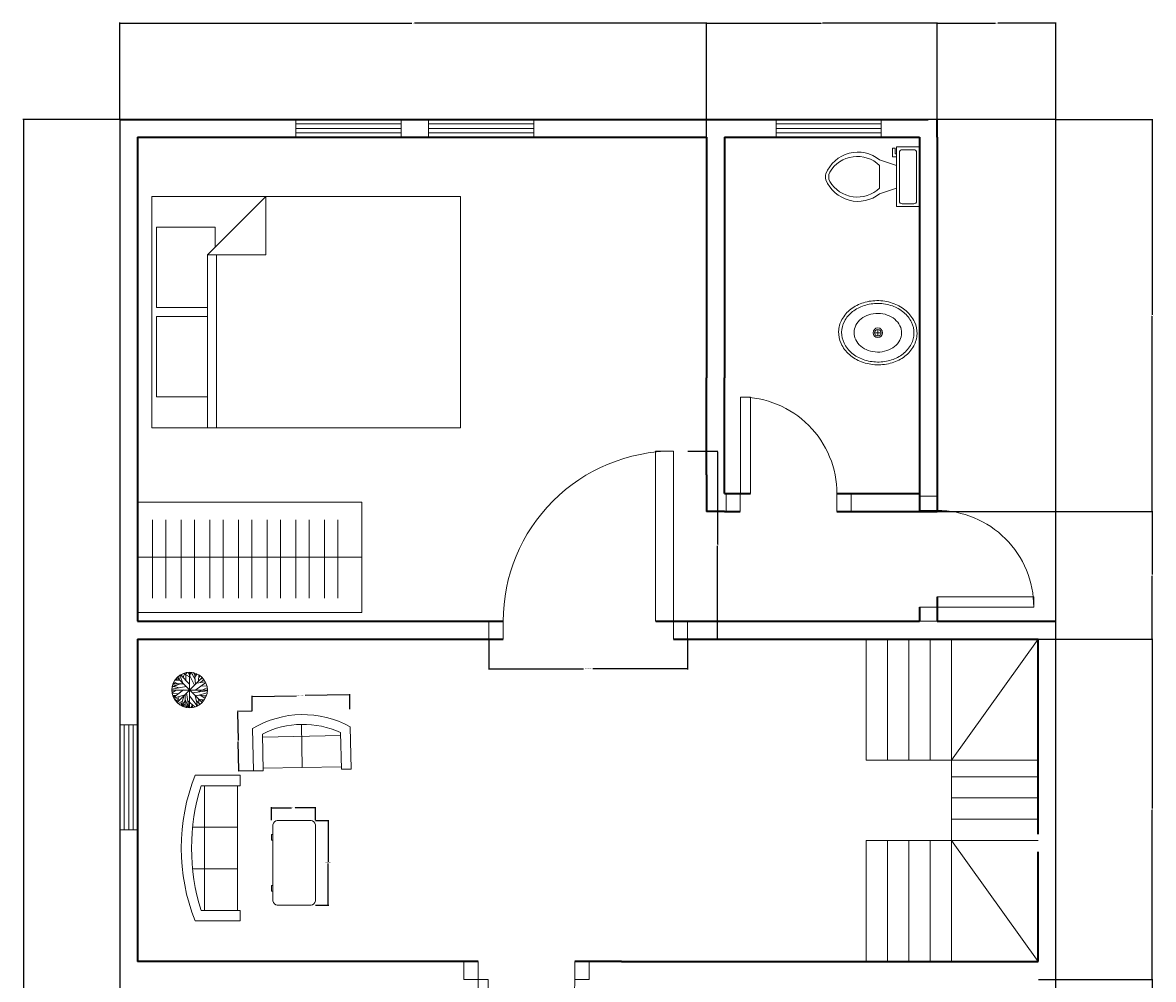
# Model space of a CAD drawing. Units: feet. Extents: x 2306 to 3052, y 829 to 1424.
# Tile 5 of 5: x 2733 to 3052, y 1154 to 1424. Entities that reach past the tile are written whole.
import ezdxf

# ---------------------------------------------------------------- set-up
doc = ezdxf.new("R2010")
doc.units = ezdxf.units.FT
for name, color, linetype, lineweight in [('A-ANNO-DIMS', 2, 'Continuous', 18), ('A-DOOR', 3, 'Continuous', 18), ('A-FLOR-FIXT', 9, 'Continuous', 18), ('A-FLOR-OTLN', 7, 'Continuous', 25), ('A-FLOR-STRS', 7, 'Continuous', 18), ('A-FURN', 8, 'Continuous', 13), ('A-GLAZ', 4, 'Continuous', 18), ('A-WALL', 7, 'Continuous', 35), ('L-PLNT', 94, 'Continuous', 13)]:
    doc.layers.add(name, color=color, linetype=linetype, lineweight=lineweight)
doc.styles.get("Standard").update_dxf_attribs({"font": 'arial.ttf'})
doc.dimstyles.get("Standard").update_dxf_attribs({"dimtxt": 0.18, "dimasz": 0.18, "dimexe": 0.18, "dimexo": 0.0625, "dimgap": 0.09, "dimtad": 0, "dimtih": 1, "dimtoh": 1, "dimdec": 4, "dimzin": 0, "dimdsep": 46, "dimlunit": 4, "dimtxsty": 'Standard', "dimcen": 0.09, "dimadec": 0, "dimazin": 0, "dimtfac": 1, "dimtdec": 4, "dimtofl": 0, "dimtmove": 0, "dimatfit": 3, "dimfxl": 1, "dimtolj": 1, "dimtzin": 0, "dimarcsym": 0})

# ---------------------------------------------------------------- blocks, each defined once
blk = doc.blocks.new('Window - Wood Frame 36 in. Wide plan')
for p, q in [((0, 6), (0, 0)), ((0, 4.5), (36, 4.5)), ((36, 6), (36, 0)), ((0, 3), (36, 3)), ((0, 1.5), (36, 1.5))]:
    blk.add_line(p, q)
blk = doc.blocks.new('Bed - Queen')
for p, q in [((0, -80.00003), (0, 0)), ((0, 0), (59.99999, 0)), ((59.99999, 0), (59.99999, -80.00003)), ((7.99999, -1.2), (28.79998, -1.2)), ((7.99999, -14.4), (7.99999, -1.2)), ((28.79998, -1.2), (28.79998, -14.4)), ((31.19999, -1.2), (51.99999, -1.2)), ((31.19999, -14.4), (31.19999, -1.2)), ((51.99999, -1.2), (51.99999, -16.4)), ((0, -14.4), (44.8, -14.4)), ((59.99999, -29.6), (44.8, -14.4)), ((44.8, -14.4), (44.8, -29.6)), ((44.8, -16.8), (0, -16.8)), ((51.99999, -16.4), (46.79936, -16.4)), ((44.8, -29.6), (59.99999, -29.6)), ((59.99999, -80.00003), (0, -80.00003))]:
    blk.add_line(p, q)
blk = doc.blocks.new('Toilet - top')
for p, q in [((9.5, -6), (9.5, -2)), ((-10, -8.5), (-8, -8.5)), ((-10, -9.5), (-10, -8.5)), ((-7, -9.5), (-10, -9.5)), ((-8, -8.5), (-8, -8)), ((-7, -8), (-7, -9.5)), ((-4, -8), (-6, -14)), ((4, -8), (6, -14)), ((4, -14), (-4, -14))]:
    blk.add_line(p, q)
blk.add_lwpolyline([(10.5, -8), (10.5, 0), (-10.5, 0), (-10.5, -8)], close=True)
for points in [[(-9.5, -2), (-9.5, -6)], [(8.5, -1), (-8.5, -1)], [(-8.5, -7), (8.5, -7)]]:
    blk.add_lwpolyline(points)
for centre, radius, start, end in [((-8.62, -1.88), 0.884, 81.8699, 188.1301), ((8.62, -1.88), 0.884, 351.8699, 98.1301), ((-8.62, -6.12), 0.884, 171.8699, 278.1301), ((8.62, -6.12), 0.884, 261.8699, 8.1301), ((3.52, -21.58), 12.17, 141.4691, 247.9714), ((4.2, -21.82), 11.33, 136.3677, 238.9468), ((-3.52, -21.58), 12.17, 292.0284, 38.5307), ((-4.2, -21.82), 11.33, 301.053, 43.6321), ((0, -27.88), 4, 245.7318, 294.2682), ((0, -29), 4, 254.8605, 285.1395)]:
    blk.add_arc(centre, radius, start, end)
blk = doc.blocks.new('Sink - Oval top')
for p, q in [((-1, 0), (1, 0)), ((0, 1), (0, -1))]:
    blk.add_line(p, q)
for points in [[(-12.23, 0.39, 0.117634), (-11.46, -3.36, 0.104469), (-8.88, -6.8, 0.090016), (-5.08, -9.07, 0.08192), (-0.32, -10.02, 0.08192), (4.49, -9.38, 0.090016), (8.42, -7.36, 0.104469), (11.22, -4.09, 0.117634), (12.23, -0.39, 0.117634), (11.46, 3.36, 0.104469), (8.88, 6.8, 0.090016), (5.08, 9.07, 0.08192), (0.32, 10.02, 0.08192), (-4.49, 9.38, 0.090016), (-8.42, 7.36, 0.104469), (-11.22, 4.09, 0.117634)], [(-11.29, 0.16, 0.118622), (-10.52, -3.25, 0.104678), (-8.07, -6.36, 0.089562), (-4.54, -8.37, 0.081185), (-0.13, -9.15, 0.081185), (4.3, -8.49, 0.089562), (7.89, -6.58, 0.104678), (10.42, -3.55, 0.118622), (11.29, -0.16, 0.118622), (10.52, 3.25, 0.104678), (8.07, 6.36, 0.089562), (4.54, 8.37, 0.081185), (0.13, 9.15, 0.081185), (-4.3, 8.49, 0.089562), (-7.89, 6.58, 0.104678), (-10.42, 3.55, 0.118622)], [(-7.42, 0.08, 0.118283), (-6.91, -2.17, 0.104607), (-5.29, -4.21, 0.089718), (-2.97, -5.53, 0.081436), (-0.07, -6.04, 0.081436), (2.84, -5.59, 0.089718), (5.2, -4.33, 0.104607), (6.86, -2.32, 0.118283), (7.42, -0.08, 0.118283), (6.91, 2.17, 0.104607), (5.29, 4.21, 0.089718), (2.97, 5.53, 0.081436), (0.07, 6.04, 0.081436), (-2.84, 5.59, 0.089718), (-5.2, 4.33, 0.104607), (-6.86, 2.32, 0.118283)]]:
    blk.add_lwpolyline(points, format="xyb", close=True)
for radius in [1.5, 1]:
    blk.add_circle((0, 0), radius)
blk = doc.blocks.new('Sofa - Roundback 7 ft.')
for p, q in [((-36.000027, -34), (-36.000027, -11.4696)), ((-12.00002, -32.4421), (-12.00003, -6.5971)), ((11.99997, -32.4421), (11.99998, -6.5971)), ((35.99998, -34), (35.99998, -11.4696)), ((-35.999844, -13.3819), (35.9998, -13.3819)), ((-36.000027, -32.4421), (35.99998, -32.4421))]:
    blk.add_line(p, q)
for points in [[(-36.000027, -34), (-42.000027, -34), (-42.000027, -8)], [(41.99998, -8), (41.99998, -34), (35.99998, -34)]]:
    blk.add_lwpolyline(points)
for centre, radius, start, end in [((0, -114.25), 114.25, 68.43141, 111.5686), ((-0.00001, -127.1968), 121.1968, 72.72033, 107.2797)]:
    blk.add_arc(centre, radius, start, end)
blk = doc.blocks.new('Sofa - Roundback Loveseat 5 ft.')
for p, q in [((0, -32.44198), (0, -5.99998)), ((-24, -33.99998), (-24, -11.46958)), ((-23.9998, -13.38178), (23.99986, -13.38178)), ((24.00004, -33.99998), (24.00004, -11.46958)), ((-24, -32.44198), (24.00004, -32.44198))]:
    blk.add_line(p, q)
for points in [[(-24, -33.99998), (-30, -33.99998), (-30, -7.99998)], [(30.00004, -7.99998), (30.00004, -33.99998), (24.00004, -33.99998)]]:
    blk.add_lwpolyline(points)
for centre, radius, start, end in [((0, -60.24998), 60.24998, 60.13715, 119.8628), ((0, -61.38438), 55.38444, 64.32083, 115.6792)]:
    blk.add_arc(centre, radius, start, end)
blk = doc.blocks.new('Desk - 30 x 60 in.')
for p, q in [((-26.999995, 0), (26.999995, 0)), ((-29.999995, -27), (-29.999995, -3)), ((29.999995, -3), (29.999995, -27)), ((26.999995, -30), (-26.999995, -30)), ((-20.000005, -30), (-20.000005, -31)), ((-20.000005, -31), (-16.000005, -31)), ((-16.000005, -31), (-16.000005, -30)), ((15.999995, -31), (15.999995, -30)), ((19.999995, -31), (15.999995, -31)), ((19.999995, -30), (19.999995, -31))]:
    blk.add_line(p, q)
for centre, start, end in [((-26.499995, -3.5), 98.1301, 171.8699), ((26.499995, -3.5), 8.130102, 81.8699), ((-26.499995, -26.5), 188.1301, 261.8699), ((26.499995, -26.5), 278.1301, 351.8699)]:
    blk.add_arc(centre, 3.535534, start, end)
blk = doc.blocks.new('Tree - deciduous plan')
for p, q in [((-43.8768, 36.4326), (-44.405, 40.2696)), ((42, 42), (-42, -42)), ((42, -42), (-42, 42)), ((-40.1797, 44.558), (-36.4825, 43.2038)), ((-37.0107, 47.0408), (-35.25, 35.5298)), ((-32.6092, 50.4264), (-23.2782, 23.5674)), ((-31.2008, 51.1035), (-0.2149, 20.1818)), ((-26.4472, 46.5894), (-26.2712, 53.8116)), ((-22.0458, 42.0753), (-16.5881, 57.6486)), ((-21.1656, 55.8436), (-0.0388, 45.0094)), ((-12.5388, 54.9406), (-7.9613, 59.4546)), ((-12.3627, 32.1443), (-12.5388, 58.7776)), ((-5.3205, 59.6806), (16.5105, 16.7963)), ((2.426, 54.9406), (-1.4472, 59.9056)), ((0, 59.9996), (0, -60)), ((0.4894, 48.6208), (3.6584, 59.6806)), ((18.2711, 35.5298), (5.419, 59.6806)), ((9.8203, 51.5549), (12.8133, 58.5516)), ((19.6795, 19.5047), (16.3344, 57.6486)), ((17.0387, 51.1035), (23.2006, 55.1666)), ((17.7429, 43.6552), (25.4894, 54.2636)), ((31.6513, 50.8778), (30.2429, 30.5643)), ((31.1232, 42.5267), (35.8767, 48.1693)), ((-59.7219, 2.8025), (-12.0106, 12.0565)), ((-32.2571, 20.6333), (-59.1937, 9.348)), ((-58.6656, 12.7336), (-35.9543, 7.5424)), ((-57.081, 17.9248), (-47.0458, 14.7649)), ((-56.0247, 20.859), (-20.8134, 20.859)), ((-54.7923, 24.4702), (-47.75, 21.0847)), ((-54.6162, -24.7335), (-20.2853, 0.0941)), ((-53.2078, 27.4044), (-40.1797, 20.859)), ((-49.8627, 32.8214), (-32.7853, 32.8214)), ((-45.8134, 38.2383), (-40.5318, 33.0471)), ((54.3626, 25.3731), (20.9119, 0.3198)), ((23.3767, 23.3417), (53.3063, 27.4044)), ((29.3626, -6.6771), (59.4682, 7.091)), ((36.2288, 25.1474), (48.9049, 35.0784)), ((37.1091, 37.1098), (46.6161, 37.5612)), ((38.5175, 13.4107), (58.2359, 13.6364)), ((-60, 0), (60, 0)), ((-59.7219, -4.8714), (-54.2641, -6.6771)), ((-45.2853, -0.1316), (-59.0177, -10.0627)), ((-58.4895, -12.3197), (-36.4825, -11.6426)), ((-57.081, -18.4138), (-45.2853, -17.9624)), ((-52.6797, -18.188), (-55.4966, -22.0251)), ((-53.2078, -27.442), (-16.7641, -16.6081)), ((-38.9472, -29.0219), (-51.4472, -30.6018)), ((-47.2219, -19.3166), (-50.2148, -26.3135)), ((-46.5177, -30.1504), (-49.5106, -33.536)), ((-32.4331, -32.4075), (-48.1021, -35.5674)), ((-43.7008, -34.6645), (-46.6937, -37.373)), ((-35.9543, -22.4765), (-44.0529, -40.5329)), ((-24.6867, -37.8244), (-38.7712, -45.7241)), ((-19.9331, -20.2194), (-28.5599, -52.721)), ((-14.6515, -36.2445), (-27.6797, -52.9467)), ((-14.8275, -15.0282), (-14.6515, -57.6865)), ((-14.6515, -32.1818), (-3.912, -59.4922)), ((-10.074, -10.0627), (-2.5036, -59.7178)), ((-6.2008, -36.2445), (17.919, -57.0094)), ((-0.0388, -19.0909), (25.8415, -53.8495)), ((9.2922, -9.1598), (59.6443, -2.8401)), ((18.6232, -18.6394), (26.7218, -53.3981)), ((18.7992, -18.6394), (57.3556, -17.2853)), ((22.8485, -36.4702), (35.3485, -48.4326)), ((26.3697, -18.4138), (58.9401, -9.8369)), ((30.419, -30.1504), (32.3556, -50.0125)), ((31.4753, -31.279), (49.6091, -33.3103)), ((38.1654, -18.188), (52.426, -29.0219)), ((41.5105, -32.6332), (46.088, -38.0501)), ((45.9119, -24.0564), (55.595, -22.2508)), ((-26.2712, -43.9185), (-34.7219, -48.6583)), ((-14.6515, -47.3041), (-25.0388, -54.3009)), ((-21.5177, -45.4984), (-19.9331, -56.1065)), ((-8.4895, -47.5298), (-11.4825, -58.5893)), ((-6.3768, -52.721), (-9.3698, -58.815)), ((8.4119, -53.1724), (3.8344, -59.4922)), ((5.9471, -46.6269), (10.5246, -58.5893)), ((24.7852, -44.8213), (23.0246, -54.978))]:
    blk.add_line(p, q)
blk.add_circle((0, 0), 60)
blk = doc.blocks.new('DOOR-SWING-WIDE')
blk.add_lwpolyline([(52, 53), (52, 5), (56, 5), (56, 0), (52, 0), (52, 5), (47, 5), (47, 53), (48, 53), (52, 53, 0.414214), (4, 5)], format="xyb")
blk.add_lwpolyline([(4, 5), (4, 0), (0, 0), (0, 5)], close=True)
blk = doc.blocks.new('DOOR-SWING-STANDARD')
blk.add_lwpolyline([(4.02, 32.25), (4.02, 5), (1.75, 5)])
blk.add_lwpolyline([(4.02, 5), (6.86, 5), (6.86, 32.25), (6.29, 32.25), (4.02, 32.25, -0.414214), (31.27, 5)], format="xyb")
for points in [[(0, 5), (0, 0), (4, 0), (4, 5)], [(31.27, 5), (31.27, 0), (35.27, 0), (35.27, 5)]]:
    blk.add_lwpolyline(points, close=True)
blk = doc.blocks.new('WARDROBE-PLAN')
for p, q in [((0, 0), (0, 63.25)), ((0, 63.25), (8.03, 63.25)), ((2.89, 63.25), (31.17, 63.25)), ((15.59, 0), (15.59, 63.25)), ((31.17, 63.25), (31.17, 0)), ((27.14, 56.53), (4.98, 56.53)), ((27.14, 52.77), (4.98, 52.77)), ((27.14, 48.44), (4.98, 48.44)), ((27.14, 44.68), (4.98, 44.68)), ((27.14, 40.35), (4.98, 40.35)), ((27.14, 36.59), (4.98, 36.59)), ((27.14, 32.26), (4.98, 32.26)), ((27.14, 28.49), (4.98, 28.49)), ((27.14, 24.17), (4.98, 24.17)), ((27.14, 20.4), (4.98, 20.4)), ((27.14, 16.08), (4.98, 16.08)), ((27.14, 12.31), (4.98, 12.31)), ((27.14, 7.99), (4.98, 7.99)), ((27.14, 4.22), (4.98, 4.22)), ((15.59, 4.22), (27.14, 4.22)), ((31.17, 0), (0, 0))]:
    blk.add_line(p, q)
blk = doc.blocks.new('*D22')
at = {"layer": 'A-ANNO-DIMS', "color": 0, "lineweight": -2, "transparency": 16777216}
for p, q in [((2864.65, 1250.26), (2864.65, 1241.75)), ((2920.65, 1250.26), (2920.65, 1241.75)), ((2864.83, 1241.93), (2891.35, 1241.93)), ((2920.47, 1241.93), (2893.96, 1241.93))]:
    blk.add_line(p, q, dxfattribs=at)
at = {"layer": 'A-ANNO-DIMS', "color": 0, "transparency": 16777216}
for points in [[(2864.83, 1241.96), (2864.83, 1241.9), (2864.65, 1241.93)], [(2920.47, 1241.96), (2920.47, 1241.9), (2920.65, 1241.93)]]:
    blk.add_solid(points, dxfattribs=at)
at = {"layer": 'Defpoints', "color": 0, "transparency": 16777216}
for p in [(2864.65, 1250.33), (2920.65, 1250.33), (2920.65, 1241.93)]:
    blk.add_point(p, dxfattribs=at)
at = {"layer": 'A-ANNO-DIMS', "color": 0, "transparency": 16777216, "insert": (2892.65, 1241.93), "char_height": 0.18, "attachment_point": 5}
blk.add_mtext('\\A1;WIDE DOOR 56 TYP.', dxfattribs=at)
blk = doc.blocks.new('*D23')
at = {"layer": 'A-ANNO-DIMS', "color": 0, "lineweight": -2, "transparency": 16777216}
for p, q in [((2920.72, 1303.33), (2929.23, 1303.33)), ((2929.05, 1303.15), (2929.05, 1277.01)), ((2929.05, 1250.51), (2929.05, 1276.65)), ((2920.72, 1250.33), (2929.23, 1250.33))]:
    blk.add_line(p, q, dxfattribs=at)
at = {"layer": 'A-ANNO-DIMS', "color": 0, "transparency": 16777216}
for points in [[(2929.02, 1303.15), (2929.08, 1303.15), (2929.05, 1303.33)], [(2929.02, 1250.51), (2929.08, 1250.51), (2929.05, 1250.33)]]:
    blk.add_solid(points, dxfattribs=at)
at = {"layer": 'Defpoints', "color": 0, "transparency": 16777216}
for p in [(2920.65, 1303.33), (2929.05, 1303.33), (2920.65, 1250.33)]:
    blk.add_point(p, dxfattribs=at)
at = {"layer": 'A-ANNO-DIMS', "color": 0, "transparency": 16777216, "insert": (2929.05, 1276.83), "char_height": 0.18, "attachment_point": 5}
blk.add_mtext('\\A1;53 TYP.', dxfattribs=at)
blk = doc.blocks.new('*D34')
at = {"layer": 'A-ANNO-DIMS', "color": 0, "lineweight": -2, "transparency": 16777216}
for p, q in [((2797.91, 1230.04), (2797.83, 1234.28)), ((2798.01, 1234.11), (2810.38, 1234.34)), ((2825.2, 1234.62), (2812.83, 1234.39)), ((2825.46, 1230.55), (2825.38, 1234.8))]:
    blk.add_line(p, q, dxfattribs=at)
at = {"layer": 'A-ANNO-DIMS', "color": 0, "transparency": 16777216}
for points in [[(2798.01, 1234.14), (2798.01, 1234.08), (2797.83, 1234.1)], [(2825.2, 1234.65), (2825.2, 1234.59), (2825.38, 1234.62)]]:
    blk.add_solid(points, dxfattribs=at)
at = {"layer": 'Defpoints', "color": 0, "transparency": 16777216}
for p in [(2825.38, 1234.62), (2797.91, 1229.97), (2825.46, 1230.49)]:
    blk.add_point(p, dxfattribs=at)
at = {"layer": 'A-ANNO-DIMS', "color": 0, "transparency": 16777216, "insert": (2811.61, 1234.36), "char_height": 0.18, "attachment_point": 5}
blk.add_mtext('\\A1;LOVESEAT 28 TYP.', dxfattribs=at)
blk = doc.blocks.new('*D35')
at = {"layer": 'A-ANNO-DIMS', "color": 0, "lineweight": -2, "transparency": 16777216}
for p, q in [((2797.85, 1229.97), (2793.6, 1229.89)), ((2793.78, 1229.72), (2793.93, 1221.66)), ((2794.09, 1213.24), (2793.94, 1221.3)), ((2798.16, 1213.14), (2793.91, 1213.06))]:
    blk.add_line(p, q, dxfattribs=at)
at = {"layer": 'A-ANNO-DIMS', "color": 0, "transparency": 16777216}
for points in [[(2793.81, 1229.72), (2793.75, 1229.71), (2793.78, 1229.9)], [(2794.12, 1213.24), (2794.06, 1213.24), (2794.09, 1213.06)]]:
    blk.add_solid(points, dxfattribs=at)
at = {"layer": 'Defpoints', "color": 0, "transparency": 16777216}
for p in [(2793.78, 1229.9), (2797.91, 1229.97), (2798.23, 1213.14)]:
    blk.add_point(p, dxfattribs=at)
at = {"layer": 'A-ANNO-DIMS', "color": 0, "transparency": 16777216, "insert": (2793.94, 1221.48), "char_height": 0.18, "attachment_point": 5}
blk.add_mtext('\\A1;17 TYP.', dxfattribs=at)
blk = doc.blocks.new('*D36')
at = {"layer": 'A-ANNO-DIMS', "color": 0, "lineweight": -2, "transparency": 16777216}
for p, q in [((2815.75, 1199.15), (2819.45, 1199.15)), ((2819.27, 1198.97), (2819.27, 1187.39)), ((2819.27, 1175.45), (2819.27, 1187.03)), ((2815.75, 1175.27), (2819.45, 1175.27))]:
    blk.add_line(p, q, dxfattribs=at)
at = {"layer": 'A-ANNO-DIMS', "color": 0, "transparency": 16777216}
for points in [[(2819.24, 1198.97), (2819.3, 1198.97), (2819.27, 1199.15)], [(2819.24, 1175.45), (2819.3, 1175.45), (2819.27, 1175.27)]]:
    blk.add_solid(points, dxfattribs=at)
at = {"layer": 'Defpoints', "color": 0, "transparency": 16777216}
for p in [(2815.69, 1199.15), (2815.69, 1175.27), (2819.27, 1175.27)]:
    blk.add_point(p, dxfattribs=at)
at = {"layer": 'A-ANNO-DIMS', "color": 0, "transparency": 16777216, "insert": (2819.27, 1187.21), "char_height": 0.18, "attachment_point": 5}
blk.add_mtext('\\A1;DESK 24 TYP.', dxfattribs=at)
blk = doc.blocks.new('*D37')
at = {"layer": 'A-ANNO-DIMS', "color": 0, "lineweight": -2, "transparency": 16777216}
for p, q in [((2803.35, 1199.22), (2803.35, 1202.92)), ((2803.53, 1202.74), (2809, 1202.74)), ((2815.51, 1202.74), (2810.04, 1202.74)), ((2815.69, 1199.22), (2815.69, 1202.92))]:
    blk.add_line(p, q, dxfattribs=at)
at = {"layer": 'A-ANNO-DIMS', "color": 0, "transparency": 16777216}
for points in [[(2803.53, 1202.77), (2803.53, 1202.71), (2803.35, 1202.74)], [(2815.51, 1202.77), (2815.51, 1202.71), (2815.69, 1202.74)]]:
    blk.add_solid(points, dxfattribs=at)
at = {"layer": 'Defpoints', "color": 0, "transparency": 16777216}
for p in [(2815.69, 1202.74), (2803.35, 1199.15), (2815.69, 1199.15)]:
    blk.add_point(p, dxfattribs=at)
at = {"layer": 'A-ANNO-DIMS', "color": 0, "transparency": 16777216, "insert": (2809.52, 1202.74), "char_height": 0.18, "attachment_point": 5}
blk.add_mtext('\\A1;12 TYP.', dxfattribs=at)
blk = doc.blocks.new('*D63')
at = {"layer": 'A-ANNO-DIMS', "color": 0, "lineweight": -2, "transparency": 16777216}
for p, q in [((2760.46, 1396.83), (2733.17, 1396.83)), ((2733.35, 1396.65), (2733.35, 1127.01)), ((2733.35, 857.01), (2733.35, 1126.65)), ((2760.46, 856.83), (2733.17, 856.83))]:
    blk.add_line(p, q, dxfattribs=at)
at = {"layer": 'A-ANNO-DIMS', "color": 0, "transparency": 16777216}
for points in [[(2733.32, 1396.65), (2733.38, 1396.65), (2733.35, 1396.83)], [(2733.32, 857.01), (2733.38, 857.01), (2733.35, 856.83)]]:
    blk.add_solid(points, dxfattribs=at)
at = {"layer": 'Defpoints', "color": 0, "transparency": 16777216}
for p in [(2733.35, 1396.83), (2760.52, 1396.83), (2760.52, 856.83)]:
    blk.add_point(p, dxfattribs=at)
at = {"layer": 'A-ANNO-DIMS', "color": 0, "transparency": 16777216, "insert": (2733.35, 1126.83), "char_height": 0.18, "attachment_point": 5}
blk.add_mtext('\\A1;540', dxfattribs=at)
blk = doc.blocks.new('*D65')
at = {"layer": 'A-ANNO-DIMS', "color": 0, "lineweight": -2, "transparency": 16777216}
for p, q in [((3019.59, 1154.33), (3051.88, 1154.33)), ((3051.7, 1154.15), (3051.7, 1080.01)), ((3051.7, 1005.51), (3051.7, 1079.65)), ((3019.59, 1005.33), (3051.88, 1005.33))]:
    blk.add_line(p, q, dxfattribs=at)
at = {"layer": 'A-ANNO-DIMS', "color": 0, "transparency": 16777216}
for points in [[(3051.67, 1154.15), (3051.73, 1154.15), (3051.7, 1154.33)], [(3051.67, 1005.51), (3051.73, 1005.51), (3051.7, 1005.33)]]:
    blk.add_solid(points, dxfattribs=at)
at = {"layer": 'Defpoints', "color": 0, "transparency": 16777216}
for p in [(3019.52, 1154.33), (3051.7, 1154.33), (3019.52, 1005.33)]:
    blk.add_point(p, dxfattribs=at)
at = {"layer": 'A-ANNO-DIMS', "color": 0, "transparency": 16777216, "insert": (3051.7, 1079.83), "char_height": 0.18, "attachment_point": 5}
blk.add_mtext('\\A1;149', dxfattribs=at)
blk = doc.blocks.new('*D66')
at = {"layer": 'A-ANNO-DIMS', "color": 0, "lineweight": -2, "transparency": 16777216}
for p, q in [((3019.59, 1250.33), (3051.88, 1250.33)), ((3051.7, 1250.15), (3051.7, 1202.51)), ((3051.7, 1154.51), (3051.7, 1202.15)), ((3019.59, 1154.33), (3051.88, 1154.33))]:
    blk.add_line(p, q, dxfattribs=at)
at = {"layer": 'A-ANNO-DIMS', "color": 0, "transparency": 16777216}
for points in [[(3051.67, 1250.15), (3051.73, 1250.15), (3051.7, 1250.33)], [(3051.67, 1154.51), (3051.73, 1154.51), (3051.7, 1154.33)]]:
    blk.add_solid(points, dxfattribs=at)
at = {"layer": 'Defpoints', "color": 0, "transparency": 16777216}
for p in [(3019.52, 1250.33), (3051.7, 1250.33), (3019.52, 1154.33)]:
    blk.add_point(p, dxfattribs=at)
at = {"layer": 'A-ANNO-DIMS', "color": 0, "transparency": 16777216, "insert": (3051.7, 1202.33), "char_height": 0.18, "attachment_point": 5}
blk.add_mtext('\\A1;96', dxfattribs=at)
blk = doc.blocks.new('*D67')
at = {"layer": 'A-ANNO-DIMS', "color": 0, "lineweight": -2, "transparency": 16777216}
for p, q in [((2991.09, 1286.33), (3051.88, 1286.33)), ((3051.7, 1286.15), (3051.7, 1268.51)), ((3051.7, 1250.51), (3051.7, 1268.15)), ((3019.59, 1250.33), (3051.88, 1250.33))]:
    blk.add_line(p, q, dxfattribs=at)
at = {"layer": 'A-ANNO-DIMS', "color": 0, "transparency": 16777216}
for points in [[(3051.67, 1286.15), (3051.73, 1286.15), (3051.7, 1286.33)], [(3051.67, 1250.51), (3051.73, 1250.51), (3051.7, 1250.33)]]:
    blk.add_solid(points, dxfattribs=at)
at = {"layer": 'Defpoints', "color": 0, "transparency": 16777216}
for p in [(2991.02, 1286.33), (3051.7, 1286.33), (3019.52, 1250.33)]:
    blk.add_point(p, dxfattribs=at)
at = {"layer": 'A-ANNO-DIMS', "color": 0, "transparency": 16777216, "insert": (3051.7, 1268.33), "char_height": 0.18, "attachment_point": 5}
blk.add_mtext('\\A1;36', dxfattribs=at)
blk = doc.blocks.new('*D68')
at = {"layer": 'A-ANNO-DIMS', "color": 0, "lineweight": -2, "transparency": 16777216}
for p, q in [((3024.59, 1396.83), (3051.88, 1396.83)), ((3051.7, 1396.65), (3051.7, 1341.76)), ((3051.7, 1286.51), (3051.7, 1341.4)), ((2991.09, 1286.33), (3051.88, 1286.33))]:
    blk.add_line(p, q, dxfattribs=at)
at = {"layer": 'A-ANNO-DIMS', "color": 0, "transparency": 16777216}
for points in [[(3051.67, 1396.65), (3051.73, 1396.65), (3051.7, 1396.83)], [(3051.67, 1286.51), (3051.73, 1286.51), (3051.7, 1286.33)]]:
    blk.add_solid(points, dxfattribs=at)
at = {"layer": 'Defpoints', "color": 0, "transparency": 16777216}
for p in [(3024.52, 1396.83), (3051.7, 1396.83), (2991.02, 1286.33)]:
    blk.add_point(p, dxfattribs=at)
at = {"layer": 'A-ANNO-DIMS', "color": 0, "transparency": 16777216, "insert": (3051.7, 1341.58), "char_height": 0.18, "attachment_point": 5}
blk.add_mtext('\\A1;110.5', dxfattribs=at)
blk = doc.blocks.new('*D69')
at = {"layer": 'A-ANNO-DIMS', "color": 0, "lineweight": -2, "transparency": 16777216}
for p, q in [((2760.52, 1396.89), (2760.52, 1424.18)), ((2760.7, 1424), (2842.89, 1424)), ((2925.84, 1424), (2843.66, 1424)), ((2926.02, 1391.89), (2926.02, 1424.18))]:
    blk.add_line(p, q, dxfattribs=at)
at = {"layer": 'A-ANNO-DIMS', "color": 0, "transparency": 16777216}
for points in [[(2760.7, 1424.03), (2760.7, 1423.97), (2760.52, 1424)], [(2925.84, 1424.03), (2925.84, 1423.97), (2926.02, 1424)]]:
    blk.add_solid(points, dxfattribs=at)
at = {"layer": 'Defpoints', "color": 0, "transparency": 16777216}
for p in [(2926.02, 1424), (2760.52, 1396.83), (2926.02, 1391.83)]:
    blk.add_point(p, dxfattribs=at)
at = {"layer": 'A-ANNO-DIMS', "color": 0, "transparency": 16777216, "insert": (2843.27, 1424), "char_height": 0.18, "attachment_point": 5}
blk.add_mtext('\\A1;165.5', dxfattribs=at)
blk = doc.blocks.new('*D70')
at = {"layer": 'A-ANNO-DIMS', "color": 0, "lineweight": -2, "transparency": 16777216}
for p, q in [((2926.02, 1391.89), (2926.02, 1424.18)), ((2926.2, 1424), (2958.3, 1424)), ((2990.84, 1424), (2958.74, 1424)), ((2991.02, 1391.89), (2991.02, 1424.18))]:
    blk.add_line(p, q, dxfattribs=at)
at = {"layer": 'A-ANNO-DIMS', "color": 0, "transparency": 16777216}
for points in [[(2926.2, 1424.03), (2926.2, 1423.97), (2926.02, 1424)], [(2990.84, 1424.03), (2990.84, 1423.97), (2991.02, 1424)]]:
    blk.add_solid(points, dxfattribs=at)
at = {"layer": 'Defpoints', "color": 0, "transparency": 16777216}
for p in [(2991.02, 1424), (2926.02, 1391.83), (2991.02, 1391.83)]:
    blk.add_point(p, dxfattribs=at)
at = {"layer": 'A-ANNO-DIMS', "color": 0, "transparency": 16777216, "insert": (2958.52, 1424), "char_height": 0.18, "attachment_point": 5}
blk.add_mtext('\\A1;65', dxfattribs=at)
blk = doc.blocks.new('*D71')
at = {"layer": 'A-ANNO-DIMS', "color": 0, "lineweight": -2, "transparency": 16777216}
for p, q in [((2991.02, 1391.89), (2991.02, 1424.18)), ((2991.2, 1424), (3007.45, 1424)), ((3024.34, 1424), (3008.1, 1424)), ((3024.52, 1396.89), (3024.52, 1424.18))]:
    blk.add_line(p, q, dxfattribs=at)
at = {"layer": 'A-ANNO-DIMS', "color": 0, "transparency": 16777216}
for points in [[(2991.2, 1424.03), (2991.2, 1423.97), (2991.02, 1424)], [(3024.34, 1424.03), (3024.34, 1423.97), (3024.52, 1424)]]:
    blk.add_solid(points, dxfattribs=at)
at = {"layer": 'Defpoints', "color": 0, "transparency": 16777216}
for p in [(3024.52, 1424), (3024.52, 1396.83), (2991.02, 1391.83)]:
    blk.add_point(p, dxfattribs=at)
at = {"layer": 'A-ANNO-DIMS', "color": 0, "transparency": 16777216, "insert": (3007.77, 1424), "char_height": 0.18, "attachment_point": 5}
blk.add_mtext('\\A1;33.5', dxfattribs=at)

msp = doc.modelspace()

# ---------------------------------------------------------------- linework, layer by layer
at = {"layer": 'A-FLOR-OTLN'}
for p, q in [((3024.523, 1396.827), (2760.523, 1396.827)), ((2760.523, 1396.827), (2760.523, 856.827)), ((3024.523, 856.827), (3024.523, 1396.827))]:
    msp.add_line(p, q, dxfattribs=at)
at = {"layer": 'A-FLOR-STRS'}
for p, q in [((2971.055, 1250.328), (2971.055, 1216.156)), ((2977.055, 1250.328), (2977.055, 1216.156)), ((2983.055, 1250.328), (2983.055, 1216.156)), ((2989.055, 1250.328), (2989.055, 1216.156)), ((2995.055, 1250.328), (2995.055, 1159.328)), ((2995.055, 1216.156), (3019.523, 1250.328)), ((2971.055, 1216.156), (3019.523, 1216.156)), ((3019.523, 1211.499), (2995.289, 1211.499)), ((3019.523, 1205.499), (2995.289, 1205.499)), ((3019.523, 1199.499), (2995.289, 1199.499)), ((3019.523, 1193.499), (2971.055, 1193.499)), ((2971.055, 1193.499), (2971.055, 1159.328)), ((2977.055, 1193.499), (2977.055, 1159.328)), ((2983.055, 1193.499), (2983.055, 1159.328)), ((2989.055, 1193.499), (2989.055, 1159.328)), ((2995.055, 1193.499), (3019.523, 1159.328))]:
    msp.add_line(p, q, dxfattribs=at)
at = {"layer": 'A-WALL'}
for p, q in [((2760.523, 1396.827), (2928.523, 1396.827)), ((2928.523, 1396.827), (2988.523, 1396.827)), ((2991.023, 1391.827), (2991.023, 1396.827)), ((2765.523, 1391.827), (2765.523, 1255.327)), ((2765.523, 1391.827), (2926.023, 1391.827)), ((2926.023, 1391.827), (2926.023, 1323.953)), ((2931.023, 1391.827), (2931.023, 1323.953)), ((2931.023, 1391.827), (2986.023, 1391.827)), ((2986.023, 1391.827), (2986.023, 1291.327)), ((2991.023, 1391.827), (2991.023, 1291.327)), ((2926.023, 1296.682), (2926.023, 1323.953)), ((2931.023, 1291.327), (2931.023, 1323.953)), ((2926.023, 1296.682), (2926.023, 1286.327)), ((2931.023, 1291.327), (2938.373, 1291.327)), ((2962.788, 1291.327), (2986.023, 1291.327)), ((2986.023, 1291.327), (2986.023, 1286.327)), ((2991.023, 1291.327), (2991.023, 1286.327)), ((2931.023, 1286.327), (2926.023, 1286.327)), ((2931.023, 1286.327), (2935.517, 1286.327)), ((2962.788, 1286.327), (2986.023, 1286.327)), ((2986.023, 1286.327), (2991.023, 1286.327)), ((2991.023, 1262.183), (2991.023, 1255.327)), ((2986.023, 1259.327), (2986.023, 1255.327)), ((2765.523, 1255.327), (2868.655, 1255.327)), ((2911.655, 1255.327), (2926.023, 1255.327)), ((2926.023, 1255.327), (2986.023, 1255.327)), ((2991.023, 1255.328), (3019.523, 1255.328)), ((3019.523, 1255.328), (3024.523, 1255.328)), ((2765.523, 1250.327), (2765.523, 1159.328)), ((2765.523, 1250.327), (2868.655, 1250.327)), ((2916.655, 1250.327), (2926.023, 1250.327)), ((2926.023, 1250.327), (2931.023, 1250.327)), ((2931.023, 1250.327), (2991.023, 1250.327)), ((2991.023, 1250.328), (3019.523, 1250.328)), ((2991.023, 1250.328), (2991.023, 1250.327)), ((3019.523, 1195.327), (3019.523, 1250.328)), ((3019.523, 1159.328), (3019.523, 1190.327)), ((2861.597, 1159.328), (2765.523, 1159.328)), ((2902.023, 1159.328), (2888.867, 1159.328)), ((2902.023, 1159.328), (3019.523, 1159.328))]:
    msp.add_line(p, q, dxfattribs=at)

# ---------------------------------------------------------------- block references
at = {"layer": 'A-DOOR'}
for name, p in [('DOOR-SWING-STANDARD', (2931.517, 1286.327)), ('DOOR-SWING-WIDE', (2864.654, 1250.327))]:
    msp.add_blockref(name, p, dxfattribs=at)
at = {"layer": 'A-DOOR', "extrusion": (0, 0, -1), "zscale": -1}
for p, rotation in [((-2986.022, 1255.328), 89.99999999999935), ((-2857.597, 1159.328), 180)]:
    msp.add_blockref('DOOR-SWING-STANDARD', p, dxfattribs=dict(at, rotation=rotation))
at = {"layer": 'A-FLOR-FIXT', "xscale": 0.8023769030949434, "yscale": 0.8023769030949434, "zscale": 0.8023769030949434, "rotation": 270}
msp.add_blockref('Toilet - top', (2986.023, 1380.709), dxfattribs=at)
at = {"layer": 'A-FLOR-FIXT', "xscale": 0.9036611704051442, "yscale": 0.9036611704051442, "zscale": 0.9036611704051442}
msp.add_blockref('Sink - Oval top', (2974.297, 1336.713), dxfattribs=at)
at = {"layer": 'A-FURN'}
for name, p, xscale, yscale, zscale, rotation in [('Bed - Queen', (2769.574, 1309.924), 1.087596012527482, 1.087596012527482, 1.087596012527482, 90), ('Sofa - Roundback Loveseat 5 ft.', (2811.707, 1229.006), 0.4591894755531337, 0.4591894755531337, 0.4591894755531337, 1.072055691872807), ('Sofa - Roundback 7 ft.', (2777.864, 1191.358), 0.4886678051459193, 0.4886678051459193, 0.4886678051459193, 90), ('Desk - 30 x 60 in.', (2815.69, 1187.209), 0.3981448877142051, 0.3981448877142051, 0.3981448877142051, 270)]:
    msp.add_blockref(name, p, dxfattribs=dict(at, xscale=xscale, yscale=yscale, zscale=zscale, rotation=rotation))
at = {"layer": 'A-FURN', "rotation": 270.0000000000005}
msp.add_blockref('WARDROBE-PLAN', (2765.522, 1288.964), dxfattribs=at)
at = {"layer": 'A-GLAZ', "xscale": 0.82338841385576, "yscale": 0.82338841385576, "zscale": 0.82338841385576}
for p in [(2810.228, 1391.887), (2847.643, 1391.887), (2945.61, 1391.887)]:
    msp.add_blockref('Window - Wood Frame 36 in. Wide plan', p, dxfattribs=at)
at = {"layer": 'A-GLAZ', "xscale": 0.82338841385576, "yscale": 0.82338841385576, "zscale": 0.82338841385576, "rotation": 90}
msp.add_blockref('Window - Wood Frame 36 in. Wide plan', (2765.523, 1196.489), dxfattribs=at)
at = {"layer": 'L-PLNT', "xscale": 0.0833333333333333, "yscale": 0.0833333333333333, "zscale": 0.0833333333333333}
msp.add_blockref('Tree - deciduous plan', (2780.239, 1235.941), dxfattribs=at)

# ---------------------------------------------------------------- dimensions: what is measured, and where the dimension line sits
at = {"layer": 'A-ANNO-DIMS'}
for base, p1, p2, override, picture, middle in [((2926.023, 1424.002), (2760.523, 1396.827), (2926.023, 1391.827), {"dimdec": 1, "dimlfac": 1, "dimrnd": 0, "dimzin": 0, "dimdsep": 46, "dimlunit": 2}, '*D69', (2843.273, 1424.002)), ((2991.023, 1424.002), (2926.023, 1391.827), (2991.023, 1391.827), {"dimdec": 0, "dimlfac": 1, "dimrnd": 0, "dimzin": 0, "dimdsep": 46, "dimlunit": 2}, '*D70', (2958.523, 1424.002)), ((3024.523, 1424.002), (2991.023, 1391.827), (3024.523, 1396.827), {"dimdec": 1, "dimlfac": 1, "dimrnd": 0, "dimzin": 0, "dimdsep": 46, "dimlunit": 2}, '*D71', (3007.773, 1424.002))]:
    dim = msp.add_linear_dim(base=base, p1=p1, p2=p2, dimstyle='Standard', override=override, dxfattribs=at)
    dim.commit()
    dim.dimension.update_dxf_attribs({"geometry": picture, "text_midpoint": middle})
for base, p1, p2, override, picture, middle in [((2733.348, 1396.827), (2760.523, 856.827), (2760.523, 1396.827), {"dimdec": 0, "dimlfac": 1, "dimrnd": 0, "dimzin": 0, "dimdsep": 46, "dimlunit": 2}, '*D63', (2733.348, 1126.827)), ((3051.698, 1396.827), (2991.023, 1286.327), (3024.523, 1396.827), {"dimdec": 1, "dimlfac": 1, "dimrnd": 0, "dimzin": 0, "dimdsep": 46, "dimlunit": 2}, '*D68', (3051.698, 1341.577)), ((3051.698, 1286.327), (3019.523, 1250.328), (2991.023, 1286.327), {"dimdec": 0, "dimlfac": 1, "dimrnd": 0, "dimzin": 0, "dimdsep": 46, "dimlunit": 2}, '*D67', (3051.698, 1268.328)), ((3051.698, 1250.328), (3019.523, 1154.328), (3019.523, 1250.328), {"dimdec": 0, "dimlfac": 1, "dimrnd": 0, "dimzin": 0, "dimdsep": 46, "dimlunit": 2}, '*D66', (3051.698, 1202.328)), ((3051.698, 1154.328), (3019.523, 1005.328), (3019.523, 1154.328), {"dimdec": 0, "dimlfac": 1, "dimrnd": 0, "dimzin": 0, "dimdsep": 46, "dimlunit": 2}, '*D65', (3051.698, 1079.828))]:
    dim = msp.add_linear_dim(base=base, p1=p1, p2=p2, angle=90, dimstyle='Standard', override=override, dxfattribs=at)
    dim.commit()
    dim.dimension.update_dxf_attribs({"geometry": picture, "text_midpoint": middle})
for base, p1, p2, angle, text, picture, middle in [((2929.055, 1303.327), (2920.655, 1250.327), (2920.655, 1303.327), 90, '<> TYP.', '*D23', (2929.055, 1276.827)), ((2825.381, 1234.62), (2797.911, 1229.973), (2825.458, 1230.488), 1.07206, 'LOVESEAT <> TYP.', '*D34', (2811.607, 1234.362)), ((2793.779, 1229.895), (2798.226, 1213.139), (2797.911, 1229.973), 91.07206, '<> TYP.', '*D35', (2793.937, 1221.478)), ((2819.273, 1175.265), (2815.69, 1199.154), (2815.69, 1175.265), 270, 'DESK <> TYP.', '*D36', (2819.273, 1187.209))]:
    dim = msp.add_linear_dim(base=base, p1=p1, p2=p2, angle=angle, text=text, dimstyle='Standard', override={"dimdec": 0, "dimlfac": 1, "dimrnd": 0, "dimzin": 0, "dimdsep": 46, "dimlunit": 2}, dxfattribs=at)
    dim.commit()
    dim.dimension.update_dxf_attribs({"geometry": picture, "text_midpoint": middle})
for base, p1, p2, text, picture, middle in [((2920.655, 1241.927), (2864.655, 1250.327), (2920.655, 1250.327), 'WIDE DOOR <> TYP.', '*D22', (2892.655, 1241.927)), ((2815.69, 1202.737), (2803.347, 1199.154), (2815.69, 1199.154), '<> TYP.', '*D37', (2809.519, 1202.737))]:
    dim = msp.add_linear_dim(base=base, p1=p1, p2=p2, text=text, dimstyle='Standard', override={"dimdec": 0, "dimlfac": 1, "dimrnd": 0, "dimzin": 0, "dimdsep": 46, "dimlunit": 2}, dxfattribs=at)
    dim.commit()
    dim.dimension.update_dxf_attribs({"geometry": picture, "text_midpoint": middle})

doc.saveas('drawing.dxf')
